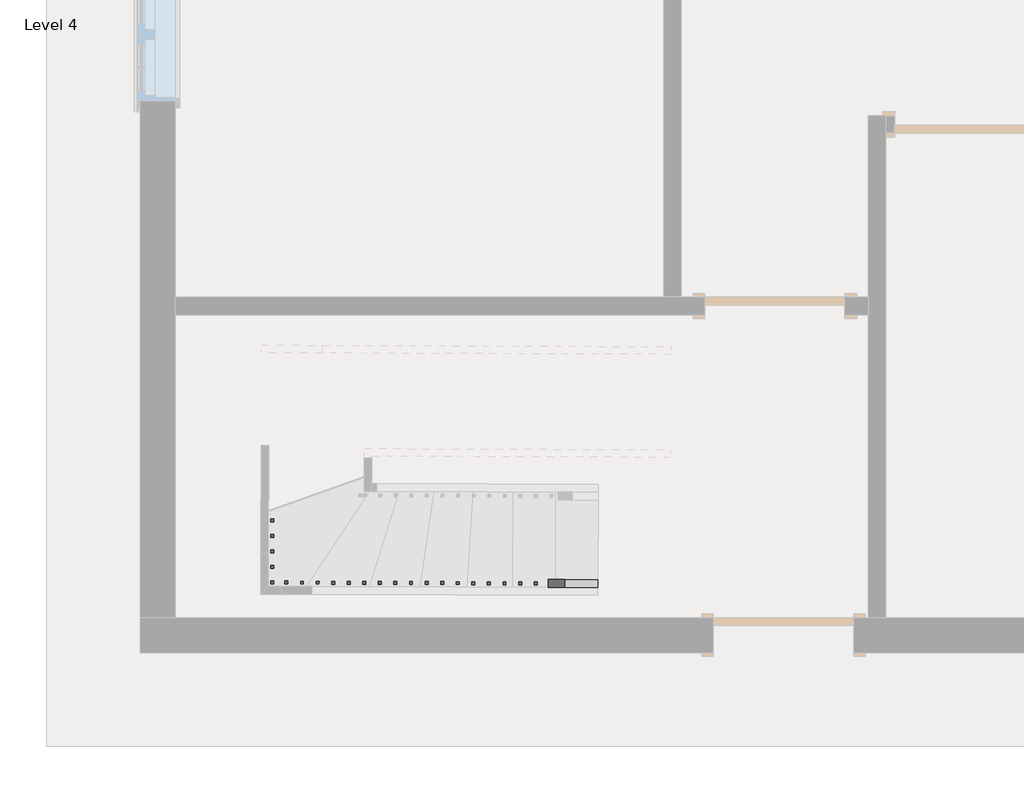
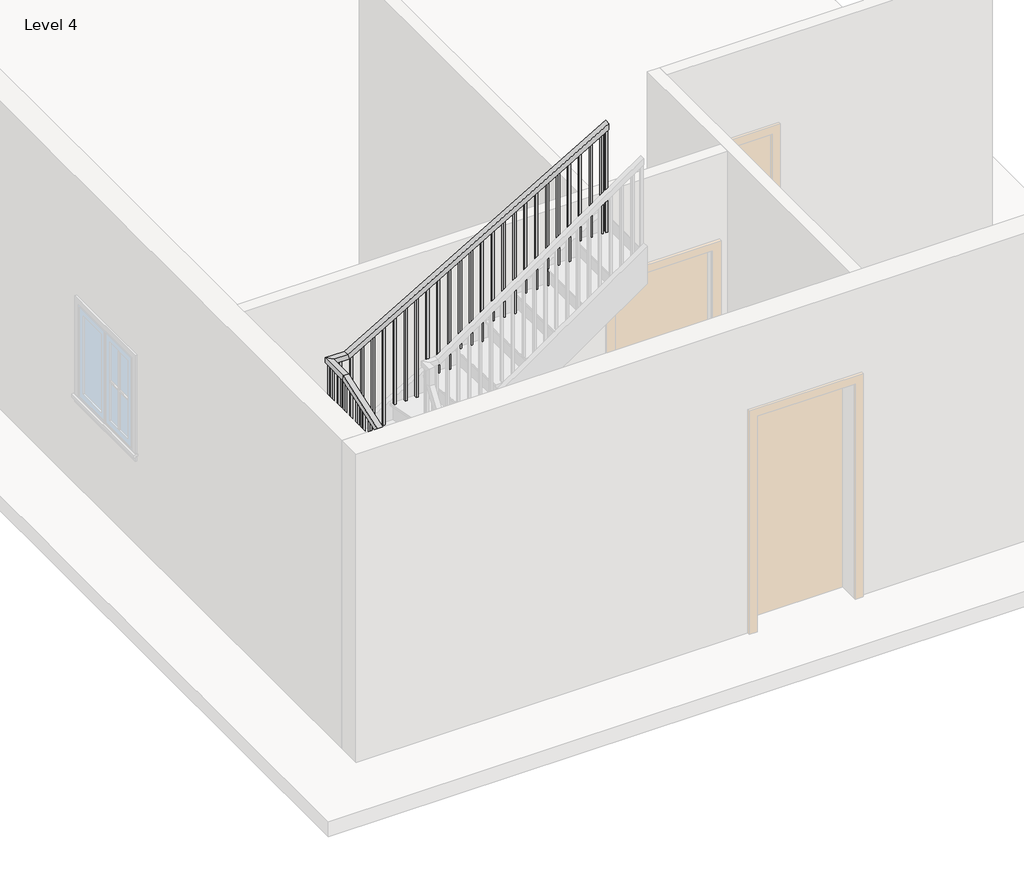
# One storey, part 2 of 3: 1 railing.
"""IFC4 building model written with IfcOpenShell, lengths in millimetres."""

from ifc_helpers import new_model, si_unit, frame, origin, place, context, project, spatial, polyline, outline, extrude, faceted_brep, element, save

model = new_model("IFC4")

# Units and contexts
model_context = context("Model", 3, world=origin())
ifc_project = project(units=[si_unit("LENGTHUNIT", "METRE", prefix="MILLI")], contexts=[model_context])

# Site, building, storey
site = spatial("IfcSite", under=ifc_project)
building = spatial("IfcBuilding", under=site)
storey = spatial("IfcBuildingStorey", under=building, Name="Level 4", Elevation=6400.8)

# Railing
placement = place(None, origin())
element("IfcRailing", 1, ObjectType="Handrail - Rectangular", at=placement, inside=storey, context=model_context, shape_type="SolidModel", body=[
    faceted_brep([(-2342.0274141, -4826.0015756, 7484.5333333), (-2342.0274141, -4826.0015756, 7426.9375993), (-2341.8555281, -4775.2018664, 7426.9375993), (-2341.8555281, -4775.2018664, 7484.5333333), (-4375.5150225, -4819.1210645, 8570.9704289), (-4388.2346185, -4819.0780265, 8520.1704289), (-4388.0627326, -4768.2783173, 8520.1704289), (-4375.3431366, -4768.3213553, 8570.9704289), (-4491.7270905, -4818.7278493, 8570.9704289), (-4491.7270905, -4818.7278493, 8520.1704289), (-4440.7554953, -4768.100026, 8520.1704289), (-4440.7554953, -4768.100026, 8570.9704289), (-4491.153576, -4649.2296115, 8570.9704289), (-4491.1254156, -4640.9069784, 8520.1704289), (-4440.3257064, -4641.0788644, 8520.1704289), (-4440.3538668, -4649.4014974, 8570.9704289), (-4487.5712496, -3590.4977417, 8927.449629), (-4487.5430892, -3582.1751086, 8876.649629), (-4436.74338, -3582.3469946, 8876.649629), (-4436.7715404, -3590.6696276, 8927.449629), (-4486.5726753, -3295.3759891, 8927.449629), (-4486.5726753, -3295.3759891, 8876.649629), (-4435.9448521, -3346.3475843, 8876.649629), (-4435.9448521, -3346.3475843, 8927.449629), (-4306.8228358, -3295.9841909, 8927.449629), (-4292.9867911, -3296.0310065, 8876.649629), (-4293.1586771, -3346.8307157, 8876.649629), (-4306.9947217, -3346.7839001, 8927.449629), (-1866.6470501, -3304.2407725, 10363.2), (-1866.8189361, -3355.0404817, 10363.2), (-1866.8189361, -3355.0404817, 10304.2591495), (-1866.6470501, -3304.2407725, 10304.2591495)], [[[0, 1, 2, 3]], [[1, 0, 4, 5]], [[2, 1, 5, 6]], [[3, 2, 6, 7]], [[0, 3, 7, 4]], [[5, 4, 8, 9]], [[6, 5, 9, 10]], [[7, 6, 10, 11]], [[4, 7, 11, 8]], [[9, 8, 12, 13]], [[10, 9, 13, 14]], [[11, 10, 14, 15]], [[8, 11, 15, 12]], [[13, 12, 16, 17]], [[14, 13, 17, 18]], [[15, 14, 18, 19]], [[12, 15, 19, 16]], [[17, 16, 20, 21]], [[18, 17, 21, 22]], [[19, 18, 22, 23]], [[16, 19, 23, 20]], [[21, 20, 24, 25]], [[22, 21, 25, 26]], [[23, 22, 26, 27]], [[20, 23, 27, 24]], [[28, 29, 30, 31]], [[25, 24, 28, 31]], [[26, 25, 31, 30]], [[27, 26, 30, 29]], [[24, 27, 29, 28]]]),
    extrude(outline(polyline([(234.2042864, 19.05), (1221.3020607, 19.05), (1221.3020607, 0.0), (222.9957135, 0.0), (234.2042864, 19.05)])), frame((-1911.7805866, -3339.0132586, 10500.7687274), z_axis=(0.0033835818014388316, 0.9999942756707125, 0.0), x_axis=(0.0, 0.0, -1.0)), (0.0, 0.0, 1.0), 19.05),
    extrude(outline(polyline([(234.2042864, 19.0499999), (1161.5230057, 19.0499999), (1161.5230057, 0.0), (222.9957136, 0.0), (234.2042864, 19.0499999)])), frame((-2013.3800051, -3338.6694867, 10440.9896724), z_axis=(0.0033835818014388316, 0.9999942756707125, 0.0), x_axis=(0.0, 0.0, -1.0)), (0.0, 0.0, 1.0), 19.05),
    extrude(outline(polyline([(234.2042864, 19.0499999), (1101.7439506, 19.0499999), (1101.7439506, 0.0), (222.9957136, 0.0), (234.2042864, 19.0499999)])), frame((-2114.9794235, -3338.3257147, 10381.2106173), z_axis=(0.0033835818014388316, 0.9999942756707125, 0.0), x_axis=(0.0, 0.0, -1.0)), (0.0, 0.0, 1.0), 19.05),
    extrude(outline(polyline([(234.2042864, 19.0499999), (1211.2982289, 19.0499999), (1211.2982289, 0.0), (222.9957135, 0.0), (234.2042864, 19.0499999)])), frame((-2216.5788419, -3337.9819428, 10321.4315622), z_axis=(0.0033835818014388316, 0.9999942756707125, 0.0), x_axis=(0.0, 0.0, -1.0)), (0.0, 0.0, 1.0), 19.05),
    extrude(outline(polyline([(234.2042864, 19.0499999), (1151.5191739, 19.0499999), (1151.5191739, 0.0), (222.9957136, 0.0), (234.2042864, 19.0499999)])), frame((-2318.1782603, -3337.6381709, 10261.6525072), z_axis=(0.0033835818014388316, 0.9999942756707125, 0.0), x_axis=(0.0, 0.0, -1.0)), (0.0, 0.0, 1.0), 19.05),
    extrude(outline(polyline([(234.2042864, 19.0499999), (1261.0734521, 19.0499999), (1261.0734521, 0.0), (222.9957136, 0.0), (234.2042864, 19.0499999)])), frame((-2419.7776787, -3337.294399, 10201.8734521), z_axis=(0.0033835818014388316, 0.9999942756707125, 0.0), x_axis=(0.0, 0.0, -1.0)), (0.0, 0.0, 1.0), 19.05),
    extrude(outline(polyline([(234.2042864, 19.0499999), (1201.294397, 19.0499999), (1201.294397, 0.0), (222.9957136, 0.0), (234.2042864, 19.0499999)])), frame((-2521.3770971, -3336.9506271, 10142.094397), z_axis=(0.0033835818014388316, 0.9999942756707125, 0.0), x_axis=(0.0, 0.0, -1.0)), (0.0, 0.0, 1.0), 19.05),
    extrude(outline(polyline([(234.2042864, 19.05), (1141.515342, 19.05), (1141.515342, 0.0), (222.9957136, 0.0), (234.2042864, 19.05)])), frame((-2622.9765155, -3336.6068552, 10082.315342), z_axis=(0.0033835818014388316, 0.9999942756707125, 0.0), x_axis=(0.0, 0.0, -1.0)), (0.0, 0.0, 1.0), 19.05),
    extrude(outline(polyline([(234.2042864, 19.05), (1251.0696202, 19.05), (1251.0696202, 0.0), (222.9957136, 0.0), (234.2042864, 19.05)])), frame((-2724.5759339, -3336.2630833, 10022.5362869), z_axis=(0.0033835818014388316, 0.9999942756707125, 0.0), x_axis=(0.0, 0.0, -1.0)), (0.0, 0.0, 1.0), 19.05),
    extrude(outline(polyline([(234.2042864, 19.05), (1191.2905651, 19.05), (1191.2905651, 0.0), (222.9957136, 0.0), (234.2042864, 19.05)])), frame((-2826.1753523, -3335.9193114, 9962.7572318), z_axis=(0.0033835818014388316, 0.9999942756707125, 0.0), x_axis=(0.0, 0.0, -1.0)), (0.0, 0.0, 1.0), 19.05),
    extrude(outline(polyline([(234.2042865, 19.05), (1131.5115101, 19.05), (1131.5115101, 0.0), (222.9957136, 0.0), (234.2042865, 19.05)])), frame((-2927.7747707, -3335.5755395, 9902.9781768), z_axis=(0.0033835818014388316, 0.9999942756707125, 0.0), x_axis=(0.0, 0.0, -1.0)), (0.0, 0.0, 1.0), 19.05),
    extrude(outline(polyline([(234.2042864, 19.05), (1241.0657884, 19.05), (1241.0657884, 0.0), (222.9957136, 0.0), (234.2042864, 19.05)])), frame((-3029.3741891, -3335.2317675, 9843.1991217), z_axis=(0.0033835818014388316, 0.9999942756707125, 0.0), x_axis=(0.0, 0.0, -1.0)), (0.0, 0.0, 1.0), 19.05),
    extrude(outline(polyline([(234.2042864, 19.05), (1181.2867333, 19.05), (1181.2867333, 0.0), (222.9957136, 0.0), (234.2042864, 19.05)])), frame((-3130.9736075, -3334.8879956, 9783.4200666), z_axis=(0.0033835818014388316, 0.9999942756707125, 0.0), x_axis=(0.0, 0.0, -1.0)), (0.0, 0.0, 1.0), 19.05),
    extrude(outline(polyline([(234.2042865, 19.0499999), (1121.5076783, 19.0499999), (1121.5076783, 0.0), (222.9957136, 0.0), (234.2042865, 19.0499999)])), frame((-3232.573026, -3334.5442237, 9723.6410116), z_axis=(0.0033835818014388316, 0.9999942756707125, 0.0), x_axis=(0.0, 0.0, -1.0)), (0.0, 0.0, 1.0), 19.05),
    extrude(outline(polyline([(234.2042864, 19.0499999), (1231.0619565, 19.0499999), (1231.0619565, 0.0), (222.9957136, 0.0), (234.2042864, 19.0499999)])), frame((-3334.1724444, -3334.2004518, 9663.8619565), z_axis=(0.0033835818014388316, 0.9999942756707125, 0.0), x_axis=(0.0, 0.0, -1.0)), (0.0, 0.0, 1.0), 19.05),
    extrude(outline(polyline([(234.2042864, 19.0499999), (1171.2829014, 19.0499999), (1171.2829014, 0.0), (222.9957136, 0.0), (234.2042864, 19.0499999)])), frame((-3435.7718628, -3333.8566799, 9604.0829014), z_axis=(0.0033835818014388316, 0.9999942756707125, 0.0), x_axis=(0.0, 0.0, -1.0)), (0.0, 0.0, 1.0), 19.05),
    extrude(outline(polyline([(234.2042864, 19.0499999), (1111.5038463, 19.0499999), (1111.5038463, 0.0), (222.9957135, 0.0), (234.2042864, 19.0499999)])), frame((-3537.3712812, -3333.512908, 9544.3038463), z_axis=(0.0033835818014388316, 0.9999942756707125, 0.0), x_axis=(0.0, 0.0, -1.0)), (0.0, 0.0, 1.0), 19.05),
    extrude(outline(polyline([(234.2042864, 19.0499999), (1221.0581246, 19.0499999), (1221.0581246, 0.0), (222.9957136, 0.0), (234.2042864, 19.0499999)])), frame((-3638.9706996, -3333.1691361, 9484.5247913), z_axis=(0.0033835818014388316, 0.9999942756707125, 0.0), x_axis=(0.0, 0.0, -1.0)), (0.0, 0.0, 1.0), 19.05),
    extrude(outline(polyline([(234.2042864, 19.0499999), (1161.2790695, 19.0499999), (1161.2790695, 0.0), (222.9957136, 0.0), (234.2042864, 19.0499999)])), frame((-3740.570118, -3332.8253642, 9424.7457362), z_axis=(0.0033835818014388316, 0.9999942756707125, 0.0), x_axis=(0.0, 0.0, -1.0)), (0.0, 0.0, 1.0), 19.05),
    extrude(outline(polyline([(234.2042864, 19.05), (1101.5000144, 19.05), (1101.5000144, 0.0), (222.9957135, 0.0), (234.2042864, 19.05)])), frame((-3842.1695364, -3332.4815923, 9364.9666811), z_axis=(0.0033835818014388316, 0.9999942756707125, 0.0), x_axis=(0.0, 0.0, -1.0)), (0.0, 0.0, 1.0), 19.05),
    extrude(outline(polyline([(234.2042864, 19.05), (1211.0542928, 19.05), (1211.0542928, 0.0), (222.9957136, 0.0), (234.2042864, 19.05)])), frame((-3943.7689548, -3332.1378203, 9305.1876261), z_axis=(0.0033835818014388316, 0.9999942756707125, 0.0), x_axis=(0.0, 0.0, -1.0)), (0.0, 0.0, 1.0), 19.05),
    extrude(outline(polyline([(234.2042864, 19.05), (1151.2752377, 19.05), (1151.2752377, 0.0), (222.9957136, 0.0), (234.2042864, 19.05)])), frame((-4045.3683732, -3331.7940484, 9245.408571), z_axis=(0.0033835818014388316, 0.9999942756707125, 0.0), x_axis=(0.0, 0.0, -1.0)), (0.0, 0.0, 1.0), 19.05),
    extrude(outline(polyline([(234.2042864, 19.05), (1091.4961826, 19.05), (1091.4961826, 0.0), (222.9957136, 0.0), (234.2042864, 19.05)])), frame((-4146.9677916, -3331.4502765, 9185.6295159), z_axis=(0.0033835818014388316, 0.9999942756707125, 0.0), x_axis=(0.0, 0.0, -1.0)), (0.0, 0.0, 1.0), 19.05),
    extrude(outline(polyline([(234.2042865, 19.05), (1031.7171276, 19.05), (1031.7171276, 0.0), (222.9957136, 0.0), (234.2042865, 19.05)])), frame((-4248.56721, -3331.1065046, 9125.8504609), z_axis=(0.0033835818014388316, 0.9999942756707125, 0.0), x_axis=(0.0, 0.0, -1.0)), (0.0, 0.0, 1.0), 19.05),
    extrude(outline(polyline([(-4369.1520622, -3311.6483845), (-4350.1021712, -3311.7128418), (-4350.1666284, -3330.7627327), (-4369.2165194, -3330.6982755), (-4369.1520622, -3311.6483845)])), frame((0.0, 0.0, 8094.1333333), z_axis=(0.0, 0.0, 1.0), x_axis=(1.0, 0.0, 0.0)), (0.0, 0.0, 1.0), 782.5162957),
    extrude(outline(polyline([(-4470.9856602, -3380.5147968), (-4470.921203, -3361.4649058), (-4451.871312, -3361.5293631), (-4451.9357693, -3380.579254), (-4470.9856602, -3380.5147968)])), frame((0.0, 0.0, 8094.1333333), z_axis=(0.0, 0.0, 1.0), x_axis=(1.0, 0.0, 0.0)), (0.0, 0.0, 1.0), 782.5162957),
    extrude(outline(polyline([(-4471.3294321, -3482.1142152), (-4471.2649749, -3463.0643242), (-4452.215084, -3463.1287815), (-4452.2795412, -3482.1786724), (-4471.3294321, -3482.1142152)])), frame((0.0, 0.0, 7924.8), z_axis=(0.0, 0.0, 1.0), x_axis=(1.0, 0.0, 0.0)), (0.0, 0.0, 1.0), 951.849629),
    extrude(outline(polyline([(-4471.6732041, -3583.7136336), (-4471.6087468, -3564.6637426), (-4452.5588559, -3564.7281999), (-4452.6233131, -3583.7780908), (-4471.6732041, -3583.7136336)])), frame((0.0, 0.0, 7924.8), z_axis=(0.0, 0.0, 1.0), x_axis=(1.0, 0.0, 0.0)), (0.0, 0.0, 1.0), 951.849629),
    extrude(outline(polyline([(231.8070867, 19.0499999), (1148.9478489, 19.0499999), (1148.9478489, 0.0), (225.3929132, 0.0), (231.8070867, 19.0499999)])), frame((-4452.9026278, -3666.3276183, 9073.7478489), z_axis=(-0.9999942756707125, 0.003383581801438912, 0.0), x_axis=(0.0, 0.0, -1.0)), (0.0, 0.0, 1.0), 19.05),
    extrude(outline(polyline([(231.8070868, 19.0499999), (1114.7389237, 19.0499999), (1114.7389237, 0.0), (225.3929133, 0.0), (231.8070868, 19.0499999)])), frame((-4453.2463997, -3767.9270367, 9039.5389237), z_axis=(-0.9999942756707125, 0.003383581801438912, 0.0), x_axis=(0.0, 0.0, -1.0)), (0.0, 0.0, 1.0), 19.05),
    extrude(outline(polyline([(231.8070867, 19.0499999), (1080.5299984, 19.0499999), (1080.5299984, 0.0), (225.3929132, 0.0), (231.8070867, 19.0499999)])), frame((-4453.5901716, -3869.5264551, 9005.3299984), z_axis=(-0.9999942756707125, 0.003383581801438912, 0.0), x_axis=(0.0, 0.0, -1.0)), (0.0, 0.0, 1.0), 19.05),
    extrude(outline(polyline([(231.8070867, 19.05), (1215.6544064, 19.05), (1215.6544064, 0.0), (225.3929132, 0.0), (231.8070867, 19.05)])), frame((-4453.9339435, -3971.1258735, 8971.1210731), z_axis=(-0.9999942756707125, 0.003383581801438912, 0.0), x_axis=(0.0, 0.0, -1.0)), (0.0, 0.0, 1.0), 19.05),
    extrude(outline(polyline([(231.8070868, 19.05), (1181.4454812, 19.05), (1181.4454812, 0.0), (225.3929133, 0.0), (231.8070868, 19.05)])), frame((-4454.2777154, -4072.7252919, 8936.9121479), z_axis=(-0.9999942756707125, 0.003383581801438912, 0.0), x_axis=(0.0, 0.0, -1.0)), (0.0, 0.0, 1.0), 19.05),
    extrude(outline(polyline([(231.8070867, 19.05), (1147.2365559, 19.05), (1147.2365559, 0.0), (225.3929132, 0.0), (231.8070867, 19.05)])), frame((-4454.6214873, -4174.3247103, 8902.7032226), z_axis=(-0.9999942756707125, 0.003383581801438912, 0.0), x_axis=(0.0, 0.0, -1.0)), (0.0, 0.0, 1.0), 19.05),
    extrude(outline(polyline([(231.8070868, 19.05), (1113.0276307, 19.05), (1113.0276307, 0.0), (225.3929133, 0.0), (231.8070868, 19.05)])), frame((-4454.9652592, -4275.9241287, 8868.4942974), z_axis=(-0.9999942756707125, 0.003383581801438912, 0.0), x_axis=(0.0, 0.0, -1.0)), (0.0, 0.0, 1.0), 19.05),
    extrude(outline(polyline([(231.8070868, 19.05), (1248.1520388, 19.05), (1248.1520388, 0.0), (225.3929133, 0.0), (231.8070868, 19.05)])), frame((-4455.3090312, -4377.5235471, 8834.2853721), z_axis=(-0.9999942756707125, 0.003383581801438912, 0.0), x_axis=(0.0, 0.0, -1.0)), (0.0, 0.0, 1.0), 19.05),
    extrude(outline(polyline([(231.8070867, 19.05), (1213.9431135, 19.05), (1213.9431135, 0.0), (225.3929132, 0.0), (231.8070867, 19.05)])), frame((-4455.6528031, -4479.1229655, 8800.0764468), z_axis=(-0.9999942756707125, 0.003383581801438912, 0.0), x_axis=(0.0, 0.0, -1.0)), (0.0, 0.0, 1.0), 19.05),
    extrude(outline(polyline([(231.8070868, 19.0499999), (1179.7341883, 19.0499999), (1179.7341883, 0.0), (225.3929133, 0.0), (231.8070868, 19.0499999)])), frame((-4455.996575, -4580.722384, 8765.8675216), z_axis=(-0.9999942756707125, 0.003383581801438912, 0.0), x_axis=(0.0, 0.0, -1.0)), (0.0, 0.0, 1.0), 19.05),
    extrude(outline(polyline([(-4475.4546951, -4701.3072361), (-4475.3902378, -4682.2573451), (-4456.3403469, -4682.3218024), (-4456.4048041, -4701.3716933), (-4475.4546951, -4701.3072361)])), frame((0.0, 0.0, 7586.1333333), z_axis=(0.0, 0.0, 1.0), x_axis=(1.0, 0.0, 0.0)), (0.0, 0.0, 1.0), 934.0370956),
    extrude(outline(polyline([(223.5110808, 19.05), (1155.0403583, 19.05), (1155.0403583, 0.0), (233.6889192, 0.0), (223.5110808, 19.05)])), frame((-4364.4371224, -4803.2834569, 8741.1736916), z_axis=(0.0033835818014387046, 0.9999942756707125, 0.0), x_axis=(0.0, 0.0, -1.0)), (0.0, 0.0, 1.0), 19.05),
    extrude(outline(polyline([(223.5110808, 19.05), (1100.7585537, 19.05), (1100.7585537, 0.0), (233.6889192, 0.0), (223.5110808, 19.05)])), frame((-4262.837704, -4803.6272288, 8686.891887), z_axis=(0.0033835818014387046, 0.9999942756707125, 0.0), x_axis=(0.0, 0.0, -1.0)), (0.0, 0.0, 1.0), 19.05),
    extrude(outline(polyline([(223.5110808, 19.05), (1215.8100824, 19.05), (1215.8100824, 0.0), (233.6889192, 0.0), (223.5110808, 19.05)])), frame((-4161.2382856, -4803.9710007, 8632.6100824), z_axis=(0.0033835818014387046, 0.9999942756707125, 0.0), x_axis=(0.0, 0.0, -1.0)), (0.0, 0.0, 1.0), 19.05),
    extrude(outline(polyline([(223.5110809, 19.0499999), (1161.5282778, 19.0499999), (1161.5282778, 0.0), (233.6889192, 0.0), (223.5110809, 19.0499999)])), frame((-4059.6388672, -4804.3147726, 8578.3282778), z_axis=(0.0033835818014387046, 0.9999942756707125, 0.0), x_axis=(0.0, 0.0, -1.0)), (0.0, 0.0, 1.0), 19.05),
    extrude(outline(polyline([(223.5110808, 19.0499999), (1107.2464731, 19.0499999), (1107.2464731, 0.0), (233.6889191, 0.0), (223.5110808, 19.0499999)])), frame((-3958.0394488, -4804.6585445, 8524.0464731), z_axis=(0.0033835818014387046, 0.9999942756707125, 0.0), x_axis=(0.0, 0.0, -1.0)), (0.0, 0.0, 1.0), 19.05),
    extrude(outline(polyline([(223.5110808, 19.0499999), (1052.9646685, 19.0499999), (1052.9646685, 0.0), (233.6889192, 0.0), (223.5110808, 19.0499999)])), frame((-3856.4400304, -4805.0023164, 8469.7646685), z_axis=(0.0033835818014387046, 0.9999942756707125, 0.0), x_axis=(0.0, 0.0, -1.0)), (0.0, 0.0, 1.0), 19.05),
    extrude(outline(polyline([(223.5110808, 19.0499999), (1168.0161972, 19.0499999), (1168.0161972, 0.0), (233.6889192, 0.0), (223.5110808, 19.0499999)])), frame((-3754.840612, -4805.3460883, 8415.4828639), z_axis=(0.0033835818014387046, 0.9999942756707125, 0.0), x_axis=(0.0, 0.0, -1.0)), (0.0, 0.0, 1.0), 19.05),
    extrude(outline(polyline([(223.5110808, 19.0499999), (1113.7343926, 19.0499999), (1113.7343926, 0.0), (233.6889192, 0.0), (223.5110808, 19.0499999)])), frame((-3653.2411936, -4805.6898602, 8361.2010593), z_axis=(0.0033835818014387046, 0.9999942756707125, 0.0), x_axis=(0.0, 0.0, -1.0)), (0.0, 0.0, 1.0), 19.05),
    extrude(outline(polyline([(223.5110808, 19.0499999), (1059.452588, 19.0499999), (1059.452588, 0.0), (233.6889192, 0.0), (223.5110808, 19.0499999)])), frame((-3551.6417752, -4806.0336322, 8306.9192547), z_axis=(0.0033835818014387046, 0.9999942756707125, 0.0), x_axis=(0.0, 0.0, -1.0)), (0.0, 0.0, 1.0), 19.05),
    extrude(outline(polyline([(223.5110808, 19.05), (1174.5041168, 19.05), (1174.5041168, 0.0), (233.6889192, 0.0), (223.5110808, 19.05)])), frame((-3450.0423567, -4806.3774041, 8252.6374501), z_axis=(0.0033835818014387046, 0.9999942756707125, 0.0), x_axis=(0.0, 0.0, -1.0)), (0.0, 0.0, 1.0), 19.05),
    extrude(outline(polyline([(223.5110809, 19.05), (1120.2223122, 19.05), (1120.2223122, 0.0), (233.6889192, 0.0), (223.5110809, 19.05)])), frame((-3348.4429383, -4806.721176, 8198.3556455), z_axis=(0.0033835818014387046, 0.9999942756707125, 0.0), x_axis=(0.0, 0.0, -1.0)), (0.0, 0.0, 1.0), 19.05),
    extrude(outline(polyline([(223.5110808, 19.05), (1065.9405075, 19.05), (1065.9405075, 0.0), (233.6889191, 0.0), (223.5110808, 19.05)])), frame((-3246.8435199, -4807.0649479, 8144.0738408), z_axis=(0.0033835818014387046, 0.9999942756707125, 0.0), x_axis=(0.0, 0.0, -1.0)), (0.0, 0.0, 1.0), 19.05),
    extrude(outline(polyline([(223.5110808, 19.05), (1180.9920362, 19.05), (1180.9920362, 0.0), (233.6889192, 0.0), (223.5110808, 19.05)])), frame((-3145.2441015, -4807.4087198, 8089.7920362), z_axis=(0.0033835818014387046, 0.9999942756707125, 0.0), x_axis=(0.0, 0.0, -1.0)), (0.0, 0.0, 1.0), 19.05),
    extrude(outline(polyline([(223.5110808, 19.05), (1126.7102316, 19.05), (1126.7102316, 0.0), (233.6889192, 0.0), (223.5110808, 19.05)])), frame((-3043.6446831, -4807.7524917, 8035.5102316), z_axis=(0.0033835818014387046, 0.9999942756707125, 0.0), x_axis=(0.0, 0.0, -1.0)), (0.0, 0.0, 1.0), 19.05),
    extrude(outline(polyline([(223.5110808, 19.05), (1072.428427, 19.05), (1072.428427, 0.0), (233.6889192, 0.0), (223.5110808, 19.05)])), frame((-2942.0452647, -4808.0962636, 7981.228427), z_axis=(0.0033835818014387046, 0.9999942756707125, 0.0), x_axis=(0.0, 0.0, -1.0)), (0.0, 0.0, 1.0), 19.05),
    extrude(outline(polyline([(223.5110808, 19.05), (1187.4799557, 19.05), (1187.4799557, 0.0), (233.6889192, 0.0), (223.5110808, 19.05)])), frame((-2840.4458463, -4808.4400355, 7926.9466224), z_axis=(0.0033835818014387046, 0.9999942756707125, 0.0), x_axis=(0.0, 0.0, -1.0)), (0.0, 0.0, 1.0), 19.05),
    extrude(outline(polyline([(223.5110809, 19.0499999), (1133.1981511, 19.0499999), (1133.1981511, 0.0), (233.6889192, 0.0), (223.5110809, 19.0499999)])), frame((-2738.8464279, -4808.7838074, 7872.6648178), z_axis=(0.0033835818014387046, 0.9999942756707125, 0.0), x_axis=(0.0, 0.0, -1.0)), (0.0, 0.0, 1.0), 19.05),
    extrude(outline(polyline([(223.5110809, 19.0499999), (1078.9163465, 19.0499999), (1078.9163465, 0.0), (233.6889192, 0.0), (223.5110809, 19.0499999)])), frame((-2637.2470095, -4809.1275794, 7818.3830132), z_axis=(0.0033835818014387046, 0.9999942756707125, 0.0), x_axis=(0.0, 0.0, -1.0)), (0.0, 0.0, 1.0), 19.05),
    extrude(outline(polyline([(223.5110808, 19.0499999), (1193.9678752, 19.0499999), (1193.9678752, 0.0), (233.6889191, 0.0), (223.5110808, 19.0499999)])), frame((-2535.6475911, -4809.4713513, 7764.1012085), z_axis=(0.0033835818014387046, 0.9999942756707125, 0.0), x_axis=(0.0, 0.0, -1.0)), (0.0, 0.0, 1.0), 19.05),
    extrude(outline(polyline([(223.5110808, 19.0499999), (1139.6860706, 19.0499999), (1139.6860706, 0.0), (233.6889192, 0.0), (223.5110808, 19.0499999)])), frame((-2434.0481727, -4809.8151232, 7709.8194039), z_axis=(0.0033835818014387046, 0.9999942756707125, 0.0), x_axis=(0.0, 0.0, -1.0)), (0.0, 0.0, 1.0), 19.05),
    extrude(outline(polyline([(-4470.8159378, -3330.3545036), (-4470.7514806, -3311.3046126), (-4451.7015896, -3311.3690698), (-4451.7660469, -3330.4189608), (-4470.8159378, -3330.3545036)])), frame((0.0, 0.0, 8094.1333333), z_axis=(0.0, 0.0, 1.0), x_axis=(1.0, 0.0, 0.0)), (0.0, 0.0, 1.0), 782.5162957),
    extrude(outline(polyline([(-4456.748576, -4802.9711117), (-4475.798467, -4802.9066545), (-4475.7340098, -4783.8567635), (-4456.6841188, -4783.9212208), (-4456.748576, -4802.9711117)])), frame((0.0, 0.0, 7586.1333333), z_axis=(0.0, 0.0, 1.0), x_axis=(1.0, 0.0, 0.0)), (0.0, 0.0, 1.0), 934.0370956),
    extrude(outline(polyline([(234.2042864, 19.05), (1247.7881964, 19.05), (1247.7881964, 0.0), (222.9957136, 0.0), (234.2042864, 19.05)])), frame((-1866.7652217, -3339.1655726, 10527.2548631), z_axis=(0.0033835818014388316, 0.9999942756707125, 0.0), x_axis=(0.0, 0.0, -1.0)), (0.0, 0.0, 1.0), 19.05),
    extrude(outline(polyline([(223.5110808, 19.05), (1090.4931852, 19.05), (1090.4931852, 0.0), (233.6889192, 0.0), (223.5110808, 19.05)])), frame((-2341.9736997, -4810.1266665, 7660.6265185), z_axis=(0.0033835818014387046, 0.9999942756707125, 0.0), x_axis=(0.0, 0.0, -1.0)), (0.0, 0.0, 1.0), 19.05),
])

save(model, "model.ifc")

# Revit data of these elements
# Type "Handrail - Rectangular"
#   Assembly Code = "C2010400"
#   built-in parameter 1008612 = 0.0416667 (stored number, unit not read)
#   built-in parameter 1008611 = 0.0416667 (stored number, unit not read)
#   built-in parameter 1008609 = 0.333333 (stored number, unit not read)
#   built-in parameter 1008604 = 0.166667 (stored number, unit not read)
#   built-in parameter 1008603 = 0.166667 (stored number, unit not read)
#   Railing Height = 3' - 0"
#   built-in parameter 1008630 = 2
#   built-in parameter 1008610 = 2
#   built-in parameter 1008618 = Baluster - Square : 3/4"
# Element 1 (IfcRailing, "Handrail - Rectangular")
#   Phase Created = New Construction
